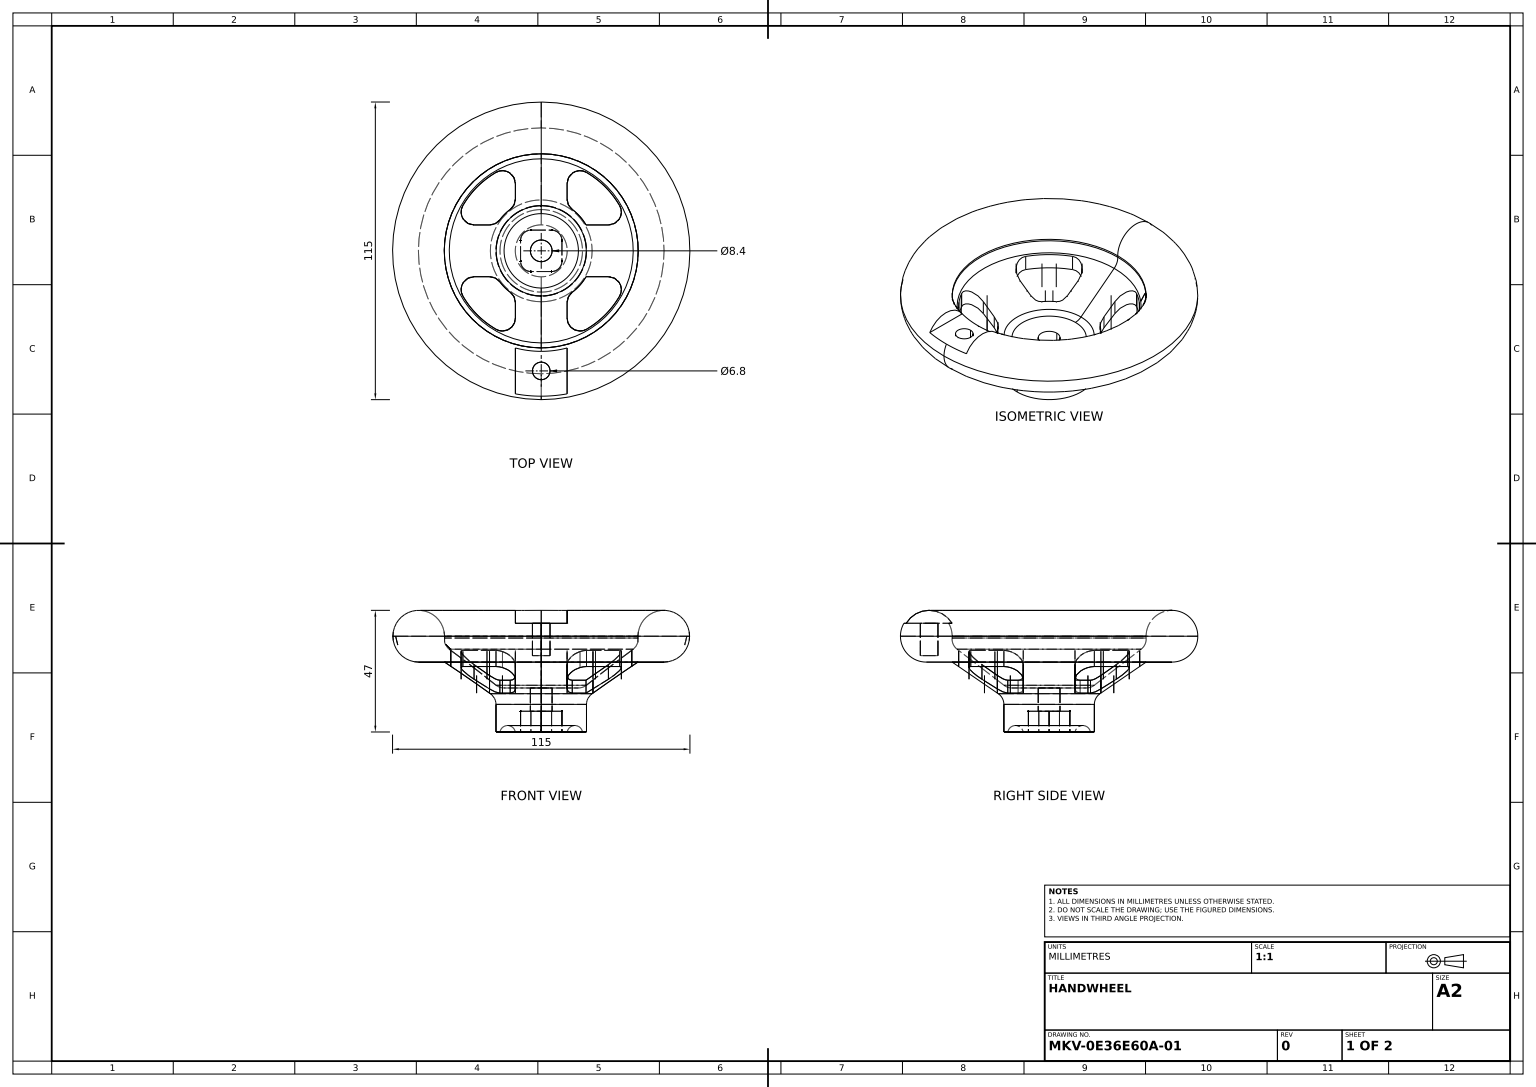
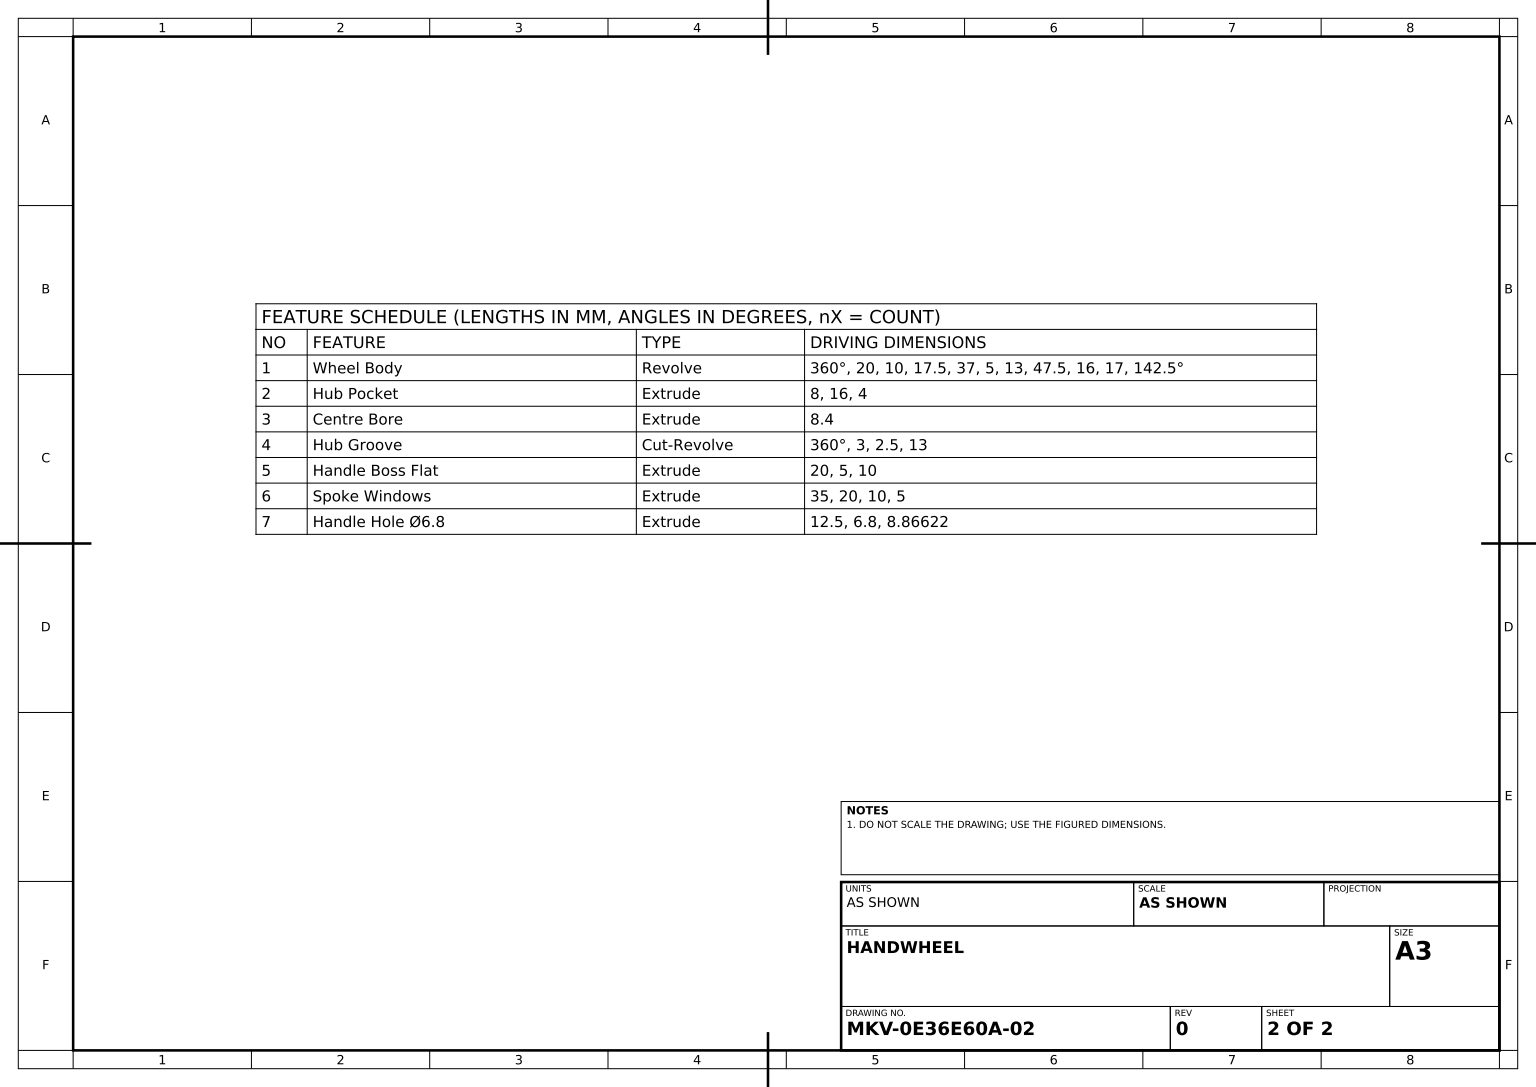
from build123d import *

# Parameters (mm, degrees)
HUB_POCKET_DEPTH          = 8
CENTRE_BORE_SKETCH_R      = 4.2
CENTRE_BORE_DEPTH         = 129.608903432
HANDLE_BOSS_FLAT_SKETCH_W = 20
HANDLE_BOSS_FLAT_SKETCH_H = 5
HANDLE_BOSS_FLAT_DEPTH    = 126.300638596
SPOKE_WINDOWS_DEPTH       = 126.300638596
HANDLE_HOLE_SKETCH_R      = 3.4
HANDLE_HOLE_6_8_DEPTH     = 12.5


with BuildPart() as part:
    # Wheel Body Profile → Wheel Body (revolve)
    with BuildSketch(Plane.XY, mode=Mode.PRIVATE) as wheel_body_sk:
        with BuildLine():
            Line((0, -10), (10, -10))
            Line((10, -10), (27.825045177, -22.206396962))
            ThreePointArc((27.825045177, -22.206396962), (29.422964271, -24), (30, -26.331820546))
            Line((30, -26.331820546), (30, -37))
            Line((30, -37), (47.5, -37))
            Line((47.5, -37), (47.5, -20))
            Line((47.5, -20), (33.108802789, -20))
            ThreePointArc((33.108802789, -20), (31.5, -19.734105363), (30.062306025, -18.964701435))
            Line((30.062306025, -18.964701435), (11.916252001, -5.021181156))
            ThreePointArc((11.916252001, -5.021181156), (10.402547886, -3.106984035), (9.975165843, -0.704319814))
            ThreePointArc((9.975165843, -0.704319814), (-6.817506944, 7.315845752), (0, -10))
        make_face()
    revolve(wheel_body_sk.sketch.rotate(Axis((47.5, -37, 0), (0, 1, 0)), 270), axis=Axis((47.5, -37, 0), (0, 1, 0)))

    # Hub Pocket Sketch → Hub Pocket (cut)
    with BuildSketch(Plane.XZ.offset(37)):
        with BuildLine():
            Line((43.5, -8), (51.5, -8))
            ThreePointArc((51.5, -8), (54.328427125, -6.828427125), (55.5, -4))
            Line((55.5, -4), (55.5, 4))
            ThreePointArc((55.5, 4), (54.328427125, 6.828427125), (51.5, 8))
            Line((51.5, 8), (43.5, 8))
            ThreePointArc((43.5, 8), (40.671572875, 6.828427125), (39.5, 4))
            Line((39.5, 4), (39.5, -4))
            ThreePointArc((39.5, -4), (40.671572875, -6.828427125), (43.5, -8))
        make_face()
    extrude(amount=-HUB_POCKET_DEPTH, mode=Mode.SUBTRACT)

    # Centre Bore Sketch → Centre Bore (cut, through all)
    with BuildSketch(Plane.XZ.offset(37)):
        with Locations(Location((47.5, 0, 0), (0, 0, 270))):
            Circle(CENTRE_BORE_SKETCH_R)
    extrude(amount=-CENTRE_BORE_DEPTH, mode=Mode.SUBTRACT)

    # Hub Groove Profile → Hub Groove (revolve, cut)
    with BuildSketch(Plane.XY, mode=Mode.PRIVATE) as hub_groove_sk:
        with BuildLine():
            Line((31.541960108, -37), (37.458039892, -37))
            ThreePointArc((37.458039892, -37), (34.5, -34.5), (31.541960108, -37))
        make_face()
    revolve(hub_groove_sk.sketch.rotate(Axis((47.5, -24.254064604, 0), (0, -1, 0)), 270), axis=Axis((47.5, -24.254064604, 0), (0, -1, 0)), mode=Mode.SUBTRACT)

    # Handle Boss Flat Sketch → Handle Boss Flat (cut, through all)
    with BuildSketch(Plane.XY):
        with Locations((47.5, 7.5)):
            Rectangle(HANDLE_BOSS_FLAT_SKETCH_W, HANDLE_BOSS_FLAT_SKETCH_H)
    extrude(amount=HANDLE_BOSS_FLAT_DEPTH, mode=Mode.SUBTRACT)

    # Spoke Windows Sketch → Spoke Windows (cut, through all)
    with BuildSketch(Plane(origin=(0, 0, 0), x_dir=(1, 0, 0), z_dir=(0, 1, 0))):
        with BuildLine():
            ThreePointArc((37.5, -20), (36.972135955, -17.763932023), (35.5, -16))
            ThreePointArc((35.5, -16), (33.357864376, -14.142135624), (31.5, -12))
            ThreePointArc((31.5, -12), (29.736067977, -10.527864045), (27.5, -10))
            Line((27.5, -10), (21.519237886, -10))
            ThreePointArc((21.519237886, -10), (17.189110868, -12.5), (17.189110868, -17.5))
            ThreePointArc((17.189110868, -17.5), (22.751262658, -24.748737342), (30, -30.310889132))
            ThreePointArc((30, -30.310889132), (35, -30.310889132), (37.5, -25.980762114))
            Line((37.5, -25.980762114), (37.5, -20))
        make_face()
        with BuildLine():
            ThreePointArc((21.519237886, 10), (17.189110868, 12.5), (17.189110868, 17.5))
            ThreePointArc((17.189110868, 17.5), (22.751262658, 24.748737342), (30, 30.310889132))
            ThreePointArc((30, 30.310889132), (35, 30.310889132), (37.5, 25.980762114))
            Line((37.5, 25.980762114), (37.5, 20))
            ThreePointArc((37.5, 20), (36.972135955, 17.763932023), (35.5, 16))
            ThreePointArc((35.5, 16), (33.357864376, 14.142135624), (31.5, 12))
            ThreePointArc((31.5, 12), (29.736067977, 10.527864045), (27.5, 10))
            Line((27.5, 10), (21.519237886, 10))
        make_face()
        with BuildLine():
            ThreePointArc((59.5, 16), (58.027864045, 17.763932023), (57.5, 20))
            Line((57.5, 20), (57.5, 25.980762114))
            ThreePointArc((57.5, 25.980762114), (60, 30.310889132), (65, 30.310889132))
            ThreePointArc((65, 30.310889132), (72.248737342, 24.748737342), (77.810889132, 17.5))
            ThreePointArc((77.810889132, 17.5), (77.810889132, 12.5), (73.480762114, 10))
            Line((73.480762114, 10), (64.820508076, 10))
            ThreePointArc((64.820508076, 10), (62.464058556, 13.269399065), (59.5, 16))
        make_face()
        with BuildLine():
            Line((73.480762114, -10), (64.820508076, -10))
            ThreePointArc((64.820508076, -10), (62.464058556, -13.269399065), (59.5, -16))
            ThreePointArc((59.5, -16), (58.027864045, -17.763932023), (57.5, -20))
            Line((57.5, -20), (57.5, -25.980762114))
            ThreePointArc((57.5, -25.980762114), (60, -30.310889132), (65, -30.310889132))
            ThreePointArc((65, -30.310889132), (72.248737342, -24.748737342), (77.810889132, -17.5))
            ThreePointArc((77.810889132, -17.5), (77.810889132, -12.5), (73.480762114, -10))
        make_face()
    extrude(amount=-SPOKE_WINDOWS_DEPTH, mode=Mode.SUBTRACT)

    # Handle Hole Sketch → Handle Hole Ø6.8 (cut)
    with BuildSketch(Plane(origin=(0, 5, 0), x_dir=(1, 0, 0), z_dir=(0, 1, 0))):
        with Locations(Location((47.5, -46.396553053, 0), (0, 0, 270))):
            Circle(HANDLE_HOLE_SKETCH_R)
    extrude(amount=-HANDLE_HOLE_6_8_DEPTH, mode=Mode.SUBTRACT)


solid = part.part
